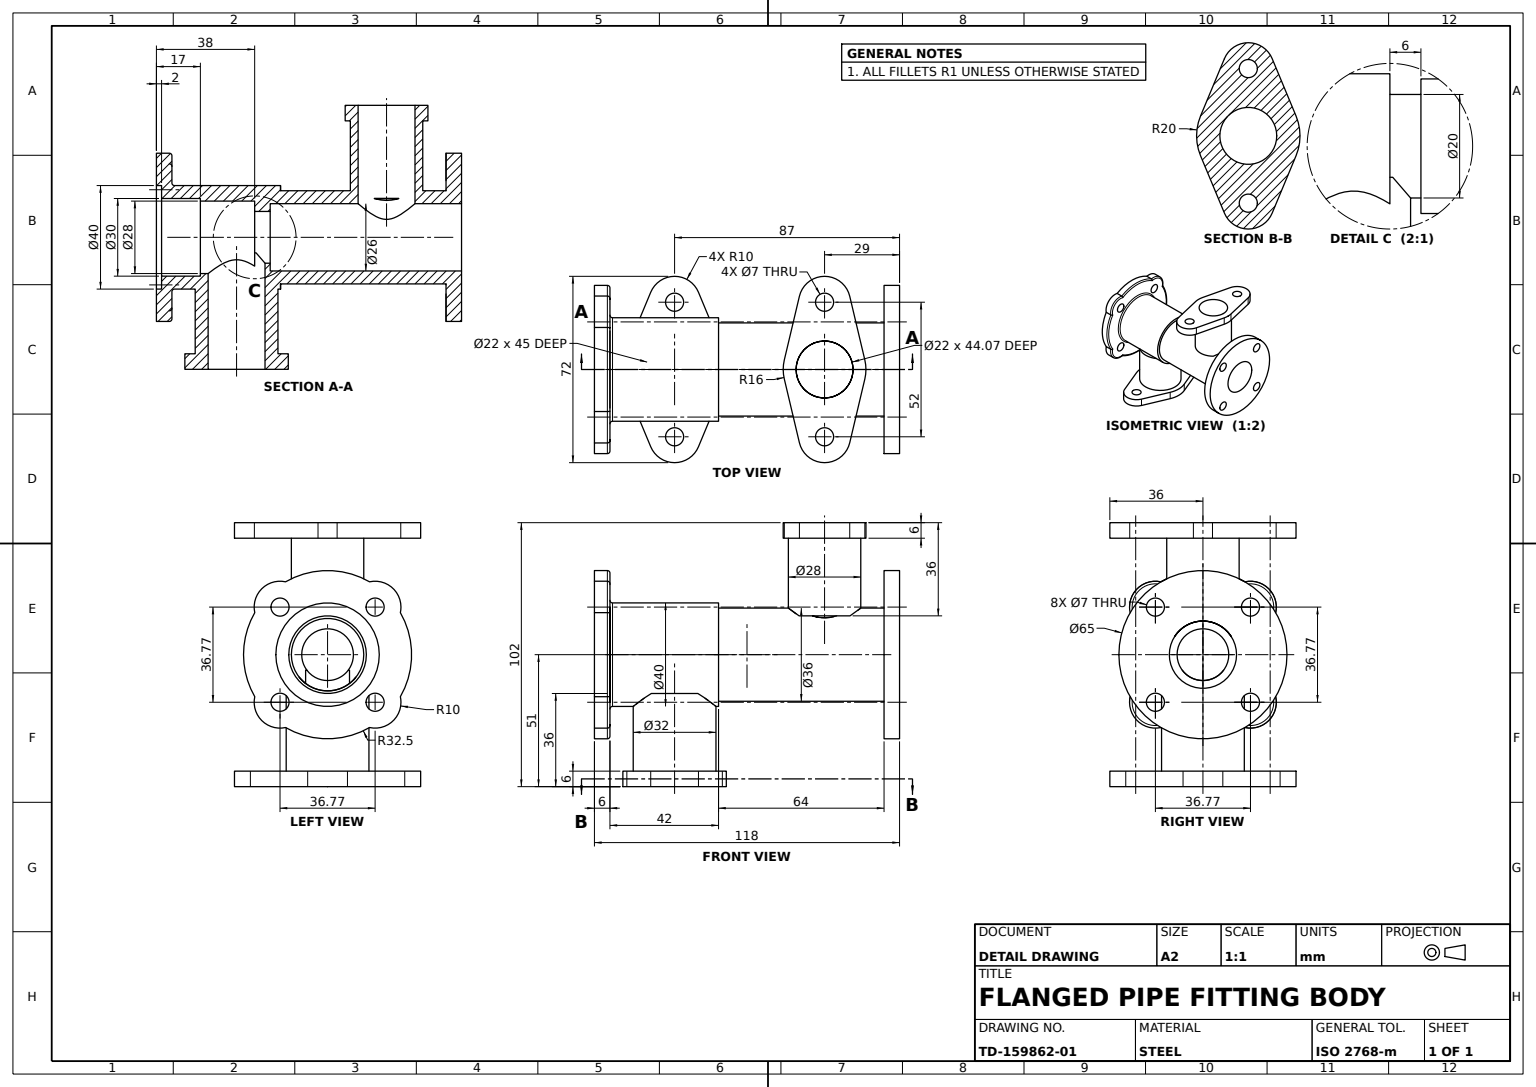
from build123d import *

# Parameters (mm, degrees)
BOTTOM_FLANGE_SKETCH_R         = 32.5
BOTTOM_FLANGE_65_DEPTH         = 6
LOWER_TUBE_SKETCH_R            = 18
LOWER_TUBE_36_DEPTH            = 64
UPPER_TUBE_SKETCH_R            = 20
UPPER_TUBE_40_DEPTH            = 42
TOP_FLANGE_SKETCH_R            = 32.5
TOP_FLANGE_65_DEPTH            = 6
TOP_START                      = -6
LOBED_PLATE_SKETCH_R           = 2.5
TOP_LOBED_PLATE_DEPTH          = 6
TOP_FLANGE_HOLES_SKETCH_R      = 3.5
TOP_FLANGE_HOLES_4X_7_DEPTH    = 6
BOTTOM_START                   = -6
BOTTOM_FLANGE_HOLES_SKETCH_R   = 3.5
BOTTOM_FLANGE_HOLES_4X_7_DEPTH = 6
TOP_START_2                    = -2
TOP_COUNTERBORE_SKETCH_R       = 20
TOP_COUNTERBORE_40_DEPTH       = 2
BORE_30_SKETCH_R               = 15
BORE_30_DEPTH                  = 15
BORE_28_SKETCH_R               = 14
BORE_28_DEPTH                  = 21
BORE_20_SKETCH_R               = 10
BORE_20_DEPTH                  = 6
BORE_26_SKETCH_R               = 13
BORE_26_DEPTH                  = 88.111996878
SIDE_PORT_1_BOSS_SKETCH_R      = 16
SIDE_PORT_1_BOSS_32_DEPTH      = 30
SIDE_PORT_1_FLANGE_DEPTH       = 6
SIDE_PORT_1_HOLES_SKETCH_R     = 3.5
SIDE_PORT_1_HOLES_2X_7_DEPTH   = 6
TOP_FLANGE_FILLET_R1_R         = 1
LOBED_PLATE_FILLET_R1_R        = 1
SIDE_PORT_1_BORE_SKETCH_R      = 11
SIDE_PORT_1_BORE_22_DEPTH      = 45
SIDE_PORT_2_BOSS_SKETCH_R      = 14
SIDE_PORT_2_BOSS_28_DEPTH      = 30
SIDE_PORT_2_FLANGE_DEPTH       = 6
SIDE_PORT_2_HOLES_SKETCH_R     = 3.5
SIDE_PORT_2_HOLES_2X_7_DEPTH   = 6
SIDE_PORT_2_BORE_SKETCH_R      = 11
SIDE_PORT_2_BORE_22_DEPTH      = 45


with BuildPart() as part:
    # Bottom Flange Sketch → Bottom Flange Ø65 (new body)
    with BuildSketch(Plane.XY):
        Circle(BOTTOM_FLANGE_SKETCH_R)
    extrude(amount=BOTTOM_FLANGE_65_DEPTH)

    # Lower Tube Sketch → Lower Tube Ø36 (add)
    with BuildSketch(Plane.XY.offset(6)):
        Circle(LOWER_TUBE_SKETCH_R)
    extrude(amount=LOWER_TUBE_36_DEPTH)

    # Upper Tube Sketch → Upper Tube Ø40 (add)
    with BuildSketch(Plane.XY.offset(70)):
        with Locations(Location((0, 0, 0), (0, 0, 180))):
            Circle(UPPER_TUBE_SKETCH_R)
    extrude(amount=UPPER_TUBE_40_DEPTH)

    # Top Flange Sketch → Top Flange Ø65 (add)
    with BuildSketch(Plane.XY.offset(112)):
        Circle(TOP_FLANGE_SKETCH_R)
    extrude(amount=TOP_FLANGE_65_DEPTH)

    # Lobed Plate Sketch → Top Lobed Plate (add)
    with BuildSketch(Plane.XY.offset(118).offset(TOP_START)):
        with BuildLine():
            ThreePointArc((-28.15193612, 16.239411711), (-22.980970389, 22.980970389), (-16.239411711, 28.15193612))
            ThreePointArc((-16.239411711, 28.15193612), (-25.455844123, 25.455844123), (-28.15193612, 16.239411711))
        make_face()
        with BuildLine():
            ThreePointArc((16.239411711, 28.15193612), (22.980970389, 22.980970389), (28.15193612, 16.239411711))
            ThreePointArc((28.15193612, 16.239411711), (25.455844123, 25.455844123), (16.239411711, 28.15193612))
        make_face()
        with BuildLine():
            ThreePointArc((16.239411711, -28.15193612), (25.455844123, -25.455844123), (28.15193612, -16.239411711))
            ThreePointArc((28.15193612, -16.239411711), (22.980970389, -22.980970389), (16.239411711, -28.15193612))
        make_face()
        with BuildLine():
            ThreePointArc((-16.239411711, -28.15193612), (-22.980970389, -22.980970389), (-28.15193612, -16.239411711))
            ThreePointArc((-28.15193612, -16.239411711), (-25.455844123, -25.455844123), (-16.239411711, -28.15193612))
        make_face()
        with Locations((-18.384776311, 18.384776311)):
            Circle(LOBED_PLATE_SKETCH_R)
        with Locations((18.384776311, 18.384776311)):
            Circle(LOBED_PLATE_SKETCH_R)
        with Locations((18.384776311, -18.384776311)):
            Circle(LOBED_PLATE_SKETCH_R)
        with Locations((-18.384776311, -18.384776311)):
            Circle(LOBED_PLATE_SKETCH_R)
    extrude(amount=TOP_LOBED_PLATE_DEPTH)

    # Top Flange Holes Sketch → Top Flange Holes 4xØ7 (cut)
    with BuildSketch(Plane.XY.offset(118)):
        with Locations((18.384776311, 18.384776311)):
            Circle(TOP_FLANGE_HOLES_SKETCH_R)
        with Locations((18.384776311, -18.384776311)):
            Circle(TOP_FLANGE_HOLES_SKETCH_R)
        with Locations((-18.384776311, -18.384776311)):
            Circle(TOP_FLANGE_HOLES_SKETCH_R)
        with Locations((-18.384776311, 18.384776311)):
            Circle(TOP_FLANGE_HOLES_SKETCH_R)
    extrude(amount=-TOP_FLANGE_HOLES_4X_7_DEPTH, mode=Mode.SUBTRACT)

    # Bottom Flange Holes Sketch → Bottom Flange Holes 4xØ7 (cut)
    with BuildSketch(Plane(origin=(0, 0, 0), x_dir=(-1, 0, 0), z_dir=(0, 0, -1)).offset(BOTTOM_START)):
        with Locations(Location((18.384776311, 18.384776311, 0), (0, 0, 180))):
            Circle(BOTTOM_FLANGE_HOLES_SKETCH_R)
        with Locations(Location((18.384776311, -18.384776311, 0), (0, 0, 180))):
            Circle(BOTTOM_FLANGE_HOLES_SKETCH_R)
        with Locations(Location((-18.384776311, -18.384776311, 0), (0, 0, 180))):
            Circle(BOTTOM_FLANGE_HOLES_SKETCH_R)
        with Locations(Location((-18.384776311, 18.384776311, 0), (0, 0, 180))):
            Circle(BOTTOM_FLANGE_HOLES_SKETCH_R)
    extrude(amount=BOTTOM_FLANGE_HOLES_4X_7_DEPTH, mode=Mode.SUBTRACT)

    # Top Counterbore Sketch → Top Counterbore Ø40 (cut)
    with BuildSketch(Plane.XY.offset(118).offset(TOP_START_2)):
        with Locations(Location((0, 0, 0), (0, 0, 180))):
            Circle(TOP_COUNTERBORE_SKETCH_R)
    extrude(amount=TOP_COUNTERBORE_40_DEPTH, mode=Mode.SUBTRACT)

    # Bore Ø30 Sketch → Bore Ø30 (cut)
    with BuildSketch(Plane.XY.offset(116)):
        Circle(BORE_30_SKETCH_R)
    extrude(amount=-BORE_30_DEPTH, mode=Mode.SUBTRACT)

    # Bore Ø28 Sketch → Bore Ø28 (cut)
    with BuildSketch(Plane.XY.offset(101)):
        Circle(BORE_28_SKETCH_R)
    extrude(amount=-BORE_28_DEPTH, mode=Mode.SUBTRACT)

    # Bore Ø20 Sketch → Bore Ø20 (cut)
    with BuildSketch(Plane.XY.offset(80)):
        Circle(BORE_20_SKETCH_R)
    extrude(amount=-BORE_20_DEPTH, mode=Mode.SUBTRACT)

    # Bore Ø26 Sketch → Bore Ø26 (cut, through all)
    with BuildSketch(Plane.XY.offset(74)):
        Circle(BORE_26_SKETCH_R)
    extrude(amount=-BORE_26_DEPTH, mode=Mode.SUBTRACT)

    # Side Port 1 Boss Sketch → Side Port 1 Boss Ø32 (add)
    with BuildSketch(Plane(origin=(0, -15, 0), x_dir=(1, 0, 0), z_dir=(0, 1, 0))):
        with Locations(Location((0, -87, 0), (0, 0, 270))):
            Circle(SIDE_PORT_1_BOSS_SKETCH_R)
    extrude(amount=-SIDE_PORT_1_BOSS_32_DEPTH)

    # Side Port 1 Flange Sketch → Side Port 1 Flange (add)
    with BuildSketch(Plane.XZ.offset(45)):
        with BuildLine():
            Line((-29.846153846, 96.230769231), (-7.692307692, 105.461538462))
            ThreePointArc((-7.692307692, 105.461538462), (0, 107), (7.692307692, 105.461538462))
            Line((7.692307692, 105.461538462), (29.846153846, 96.230769231))
            ThreePointArc((29.846153846, 96.230769231), (36, 87), (29.846153846, 77.769230769))
            Line((29.846153846, 77.769230769), (7.692307692, 68.538461538))
            ThreePointArc((7.692307692, 68.538461538), (0, 67), (-7.692307692, 68.538461538))
            Line((-7.692307692, 68.538461538), (-29.846153846, 77.769230769))
            ThreePointArc((-29.846153846, 77.769230769), (-36, 87), (-29.846153846, 96.230769231))
        make_face()
    extrude(amount=SIDE_PORT_1_FLANGE_DEPTH)

    # Side Port 1 Holes Sketch → Side Port 1 Holes 2xØ7 (cut)
    with BuildSketch(Plane.XZ.offset(51)):
        with Locations(Location((-26, 87, 0), (0, 0, 270))):
            Circle(SIDE_PORT_1_HOLES_SKETCH_R)
        with Locations(Location((26, 87, 0), (0, 0, 270))):
            Circle(SIDE_PORT_1_HOLES_SKETCH_R)
    extrude(amount=-SIDE_PORT_1_HOLES_2X_7_DEPTH, mode=Mode.SUBTRACT)

    # Top Flange Fillet R1
    top_flange_fillet_r1_edges = [part.edges().sort_by_distance(p)[0] for p in [
        (20, 0, 112),
    ]]
    fillet(top_flange_fillet_r1_edges, radius=TOP_FLANGE_FILLET_R1_R)

    # Lobed Plate Fillet R1
    lobed_plate_fillet_r1_edges = [part.edges().sort_by_distance(p)[0] for p in [
        (-32.5, 0, 112),
        (-25.455844123, 25.455844123, 112),
        (0, 32.5, 112),
        (25.455844123, 25.455844123, 112),
        (32.5, 0, 112),
        (25.455844123, -25.455844123, 112),
        (0, -32.5, 112),
        (-25.455844123, -25.455844123, 112),
    ]]
    fillet(lobed_plate_fillet_r1_edges, radius=LOBED_PLATE_FILLET_R1_R)

    # Side Port 1 Bore Sketch → Side Port 1 Bore Ø22 (cut)
    with BuildSketch(Plane.XZ.offset(51)):
        with Locations(Location((0, 87, 0), (0, 0, 270))):
            Circle(SIDE_PORT_1_BORE_SKETCH_R)
    extrude(amount=-SIDE_PORT_1_BORE_22_DEPTH, mode=Mode.SUBTRACT)

    # Side Port 2 Boss Sketch → Side Port 2 Boss Ø28 (add)
    with BuildSketch(Plane(origin=(0, 15, 0), x_dir=(1, 0, 0), z_dir=(0, 1, 0))):
        with Locations(Location((0, -29, 0), (0, 0, 44.707669521))):
            Circle(SIDE_PORT_2_BOSS_SKETCH_R)
    extrude(amount=SIDE_PORT_2_BOSS_28_DEPTH)

    # Side Port 2 Flange Sketch → Side Port 2 Flange (add)
    with BuildSketch(Plane(origin=(0, 45, 0), x_dir=(1, 0, 0), z_dir=(0, 1, 0))):
        with BuildLine():
            Line((-28.307692308, -19.269914892), (-3.692307692, -13.431863827))
            ThreePointArc((-3.692307692, -13.431863827), (0, -13), (3.692307692, -13.431863827))
            Line((3.692307692, -13.431863827), (28.307692308, -19.269914892))
            ThreePointArc((28.307692308, -19.269914892), (36, -29), (28.307692308, -38.730085108))
            Line((28.307692308, -38.730085108), (3.692307692, -44.568136173))
            ThreePointArc((3.692307692, -44.568136173), (0, -45), (-3.692307692, -44.568136173))
            Line((-3.692307692, -44.568136173), (-28.307692308, -38.730085108))
            ThreePointArc((-28.307692308, -38.730085108), (-36, -29), (-28.307692308, -19.269914892))
        make_face()
    extrude(amount=SIDE_PORT_2_FLANGE_DEPTH)

    # Side Port 2 Holes Sketch → Side Port 2 Holes 2xØ7 (cut)
    with BuildSketch(Plane(origin=(0, 51, 0), x_dir=(1, 0, 0), z_dir=(0, 1, 0))):
        with Locations(Location((-26, -29, 0), (0, 0, 270))):
            Circle(SIDE_PORT_2_HOLES_SKETCH_R)
        with Locations(Location((26, -29, 0), (0, 0, 270))):
            Circle(SIDE_PORT_2_HOLES_SKETCH_R)
    extrude(amount=-SIDE_PORT_2_HOLES_2X_7_DEPTH, mode=Mode.SUBTRACT)

    # Side Port 2 Bore Sketch → Side Port 2 Bore Ø22 (cut)
    with BuildSketch(Plane(origin=(0, 51, 0), x_dir=(1, 0, 0), z_dir=(0, 1, 0))):
        with Locations(Location((0, -29, 0), (0, 0, 270))):
            Circle(SIDE_PORT_2_BORE_SKETCH_R)
    extrude(amount=-SIDE_PORT_2_BORE_22_DEPTH, mode=Mode.SUBTRACT)


solid = part.part
